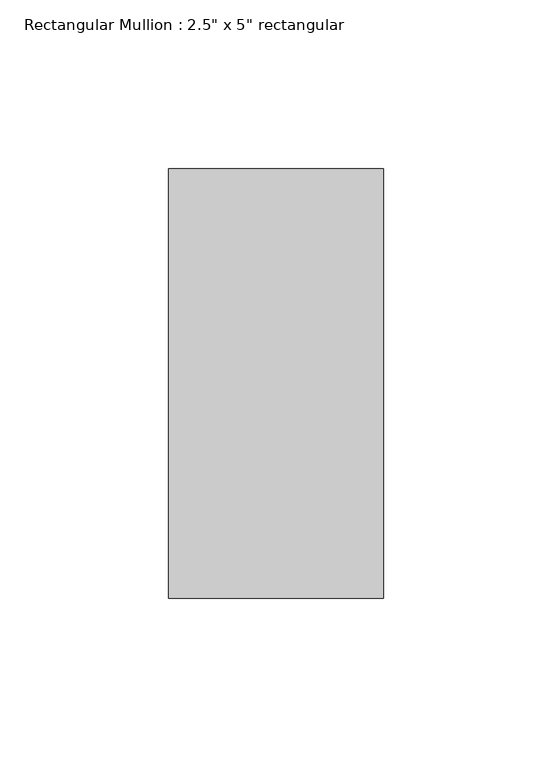
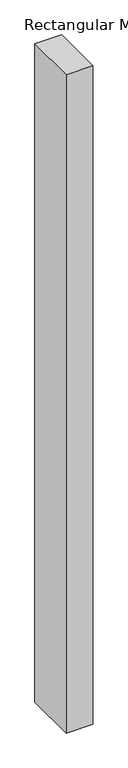
"""IFC4 building model written with IfcOpenShell, lengths in millimetres: member geometry."""

from ifc_helpers import new_model, si_unit, frame, origin, place, context, project, spatial, polyline, outline, extrude, source, transform, mapped, element, save


def member_c9d9dd2f(model_context):
    return source(origin(), model_context, "Body", "SweptSolid", [
        extrude(outline(polyline([(31.75, 63.5), (31.75, -63.5), (-31.75, -63.5), (-31.75, 63.5), (31.75, 63.5)])), frame((0.0, 0.0, -1639.8191133), z_axis=(0.0, 0.0, 1.0), x_axis=(1.0, 0.0, 0.0)), (0.0, 0.0, 1.0), 1639.8191133),
    ])


if __name__ == "__main__":
    model = new_model("IFC4")
    model_context = context("Model", 3, world=origin())
    ifc_project = project(units=[si_unit("LENGTHUNIT", "METRE", prefix="MILLI")], contexts=[model_context])
    site = spatial("IfcSite", under=ifc_project)
    building = spatial("IfcBuilding", under=site)
    placement = place(None, origin())
    member_shape = member_c9d9dd2f(model_context)
    element("IfcMember", 1, ObjectType="Rectangular Mullion : 2.5\" x 5\" rectangular", at=placement, inside=building, context=model_context, shape_type="MappedRepresentation", body=[
        mapped(member_shape, transform((0.0, 0.0, 0.0), x_axis=(1.0, 0.0, 0.0), y_axis=(0.0, 1.0, 0.0), z_axis=(0.0, 0.0, 1.0))),
    ])
    save(model, "model.ifc")

# Revit data of these elements
# Type "Rectangular Mullion : 2.5\" x 5\" rectangular"
#   built-in parameter 1007304 = 0.416667 (stored number, unit not read)
#   built-in parameter 1007301 = 0.104167 (stored number, unit not read)
#   built-in parameter 1007300 = 0.104167 (stored number, unit not read)
# Element 1 (IfcMember, "Rectangular Mullion : 2.5\" x 5\" rectangular")
#   Materials on its faces: "Aluminum"
# Materials
#   "Aluminum": class "Metal", colour RGB 247 247 247, transparency 0, Description = "Aluminum 6061", Cost = 0
